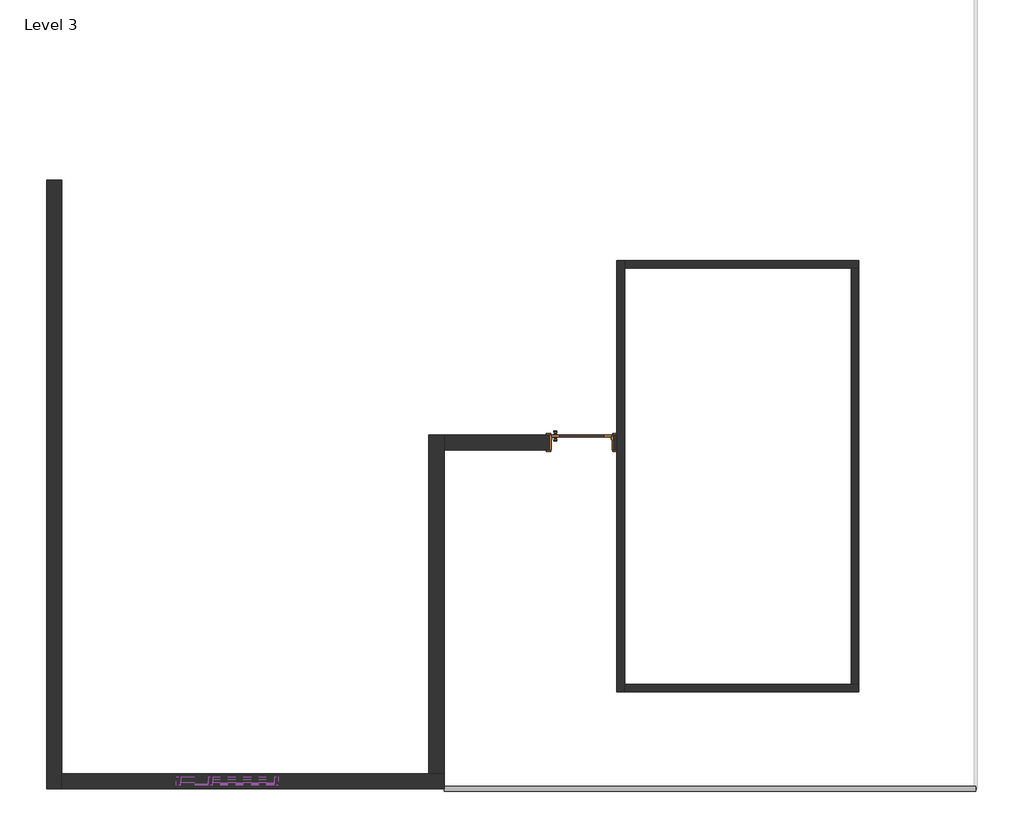
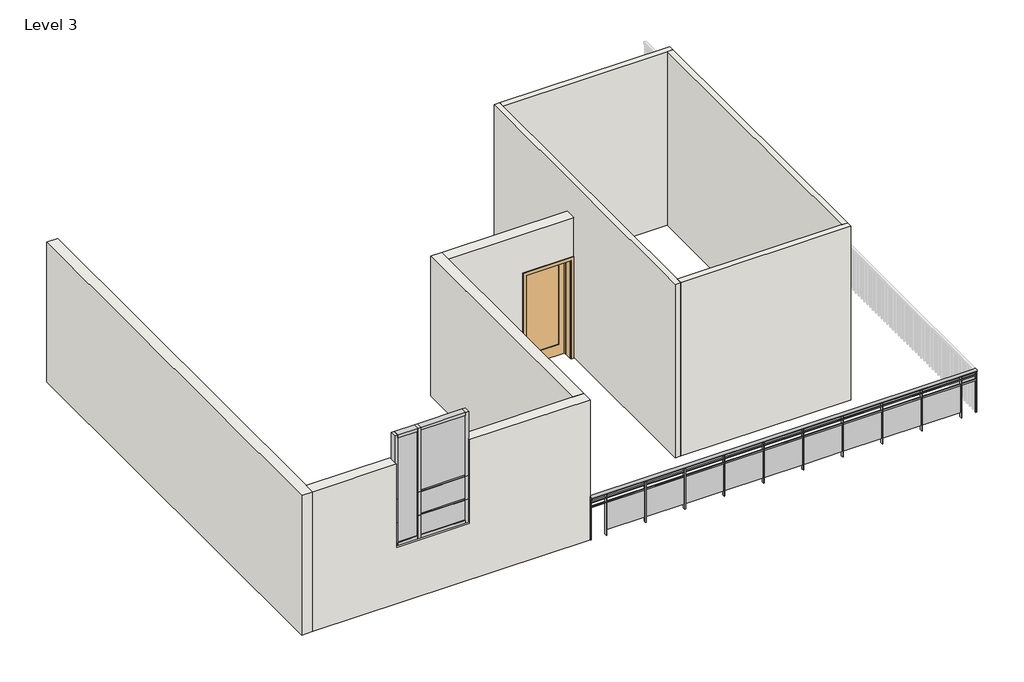
# One storey, part 1 of 2: 15 members, 8 walls, 4 plates, 1 door, 1 railing.
"""IFC4 building model written with IfcOpenShell, lengths in millimetres."""

from ifc_helpers import new_model, si_unit, point, frame, origin, place, context, project, spatial, polyline, ellipse_curve, trimmed, outline, extrude, faceted_brep, transform, mapped, element, save
from ifc_brep_helpers import plane_surface, extruded_surface, advanced_brep
from components import door_interior_single_1_panel_wood_4_x7_3b97b8e7, member_c9b54d35, member_90750a43, member_dc106669, member_ff82125d, member_7fd687a9, member_07d47f19, member_f07b7441, system_panel_glazed_5efa86ec, system_panel_glazed_31531e99, system_panel_glazed_01ea813e, system_panel_glazed_2f0fbb7d

model = new_model("IFC4")

# Units and contexts
model_context = context("Model", 3, world=origin())
ifc_project = project(units=[si_unit("LENGTHUNIT", "METRE", prefix="MILLI")], contexts=[model_context])

# Site, building, storey
site = spatial("IfcSite", under=ifc_project)
building = spatial("IfcBuilding", under=site)
storey = spatial("IfcBuildingStorey", under=building, Name="Level 3", Elevation=3810.0)

# Door
placement = place(None, origin())
door_interior_single_1_panel_wood_4_x7_shape = door_interior_single_1_panel_wood_4_x7_3b97b8e7(model_context)
element("IfcDoor", 1, ObjectType="Door-Interior-Single-1_Panel-Wood : 4'x7'", at=placement, inside=storey, context=model_context, shape_type="MappedRepresentation", body=[
    mapped(door_interior_single_1_panel_wood_4_x7_shape, transform((-360.5243879, 2041.5435469, 3810.0), x_axis=(1.0, 0.0, 0.0), y_axis=(0.0, 1.0, 0.0), z_axis=(0.0, 0.0, 1.0))),
])

# Members
member_shape = member_c9b54d35(model_context)
element("IfcMember", 2, ObjectType="Rectangular Mullion : 1.5\" x 2.5\" rectangular", at=placement, inside=storey, context=model_context, shape_type="MappedRepresentation", body=[
    mapped(member_shape, transform((-5878.6743879, -3029.0883122, 6045.2), x_axis=(0.0, 0.0, 1.0), y_axis=(0.0, 1.0, 0.0), z_axis=(-1.0, 0.0, 0.0))),
])
element("IfcMember", 3, ObjectType="Rectangular Mullion : 1.5\" x 2.5\" rectangular", at=placement, inside=storey, context=model_context, shape_type="MappedRepresentation", body=[
    mapped(member_shape, transform((-5878.6743879, -3029.0883122, 5537.2), x_axis=(0.0, 0.0, 1.0), y_axis=(0.0, 1.0, 0.0), z_axis=(-1.0, 0.0, 0.0))),
])
member_2_shape = member_90750a43(model_context)
element("IfcMember", 4, ObjectType="Rectangular Mullion : 2.5\" x 5\" rectangular", at=placement, inside=storey, context=model_context, shape_type="MappedRepresentation", body=[
    mapped(member_2_shape, transform((-5910.4243879, -3029.0883122, 5537.2), x_axis=(-1.0, 0.0, 0.0), y_axis=(0.0, 1.0, 0.0), z_axis=(0.0, 0.0, -1.0))),
])
element("IfcMember", 5, ObjectType="Rectangular Mullion : 2.5\" x 5\" rectangular", at=placement, inside=storey, context=model_context, shape_type="MappedRepresentation", body=[
    mapped(member_2_shape, transform((-5910.4243879, -3029.0883122, 5029.2), x_axis=(-1.0, 0.0, 0.0), y_axis=(0.0, 1.0, 0.0), z_axis=(0.0, 0.0, -1.0))),
])
member_3_shape = member_dc106669(model_context)
element("IfcMember", 6, ObjectType="Rectangular Mullion : 2.5\" x 5\" rectangular", at=placement, inside=storey, context=model_context, shape_type="MappedRepresentation", body=[
    mapped(member_3_shape, transform((-6354.9243879, -3029.0883122, 7442.2), x_axis=(0.0, 0.0, 1.0), y_axis=(0.0, 1.0, 0.0), z_axis=(-1.0, 0.0, 0.0))),
])
member_4_shape = member_ff82125d(model_context)
element("IfcMember", 7, ObjectType="Rectangular Mullion : 2.5\" x 5\" rectangular", at=placement, inside=storey, context=model_context, shape_type="MappedRepresentation", body=[
    mapped(member_4_shape, transform((-4957.9243879, -3029.0883122, 5029.2), x_axis=(0.0, 0.0, -1.0), y_axis=(0.0, 1.0, 0.0), z_axis=(1.0, 0.0, 0.0))),
])
element("IfcMember", 8, ObjectType="Rectangular Mullion : 2.5\" x 5\" rectangular", at=placement, inside=storey, context=model_context, shape_type="MappedRepresentation", body=[
    mapped(member_3_shape, transform((-5942.1743879, -3029.0883122, 5029.2), x_axis=(0.0, 0.0, -1.0), y_axis=(0.0, 1.0, 0.0), z_axis=(1.0, 0.0, 0.0))),
])
element("IfcMember", 9, ObjectType="Rectangular Mullion : 2.5\" x 5\" rectangular", at=placement, inside=storey, context=model_context, shape_type="MappedRepresentation", body=[
    mapped(member_4_shape, transform((-5878.6743879, -3029.0883122, 7442.2), x_axis=(0.0, 0.0, 1.0), y_axis=(0.0, 1.0, 0.0), z_axis=(-1.0, 0.0, 0.0))),
])
member_5_shape = member_7fd687a9(model_context)
element("IfcMember", 10, ObjectType="Rectangular Mullion : 2.5\" x 5\" rectangular", at=placement, inside=storey, context=model_context, shape_type="MappedRepresentation", body=[
    mapped(member_5_shape, transform((-6418.4243879, -3029.0883122, 5029.2), x_axis=(-1.0, 0.0, 0.0), y_axis=(0.0, 1.0, 0.0), z_axis=(0.0, 0.0, -1.0))),
])
element("IfcMember", 11, ObjectType="Rectangular Mullion : 2.5\" x 5\" rectangular", at=placement, inside=storey, context=model_context, shape_type="MappedRepresentation", body=[
    mapped(member_5_shape, transform((-6418.4243879, -3029.0883122, 5537.2), x_axis=(-1.0, 0.0, 0.0), y_axis=(0.0, 1.0, 0.0), z_axis=(0.0, 0.0, -1.0))),
])
element("IfcMember", 12, ObjectType="Rectangular Mullion : 2.5\" x 5\" rectangular", at=placement, inside=storey, context=model_context, shape_type="MappedRepresentation", body=[
    mapped(member_5_shape, transform((-4894.4243879, -3029.0883122, 6045.2), x_axis=(1.0, 0.0, 0.0), y_axis=(0.0, 1.0, 0.0), z_axis=(0.0, 0.0, 1.0))),
])
element("IfcMember", 13, ObjectType="Rectangular Mullion : 2.5\" x 5\" rectangular", at=placement, inside=storey, context=model_context, shape_type="MappedRepresentation", body=[
    mapped(member_5_shape, transform((-4894.4243879, -3029.0883122, 5537.2), x_axis=(1.0, 0.0, 0.0), y_axis=(0.0, 1.0, 0.0), z_axis=(0.0, 0.0, 1.0))),
])
member_6_shape = member_07d47f19(model_context)
element("IfcMember", 14, ObjectType="Rectangular Mullion : 2.5\" x 5\" rectangular", at=placement, inside=storey, context=model_context, shape_type="MappedRepresentation", body=[
    mapped(member_6_shape, transform((-5910.4243879, -3029.0883122, 6045.2), x_axis=(-1.0, 0.0, 0.0), y_axis=(0.0, 1.0, 0.0), z_axis=(0.0, 0.0, -1.0))),
])
member_7_shape = member_f07b7441(model_context)
element("IfcMember", 15, ObjectType="Rectangular Mullion : 2.5\" x 5\" rectangular", at=placement, inside=storey, context=model_context, shape_type="MappedRepresentation", body=[
    mapped(member_7_shape, transform((-4894.4243879, -3029.0883122, 7442.2), x_axis=(1.0, 0.0, 0.0), y_axis=(0.0, 1.0, 0.0), z_axis=(0.0, 0.0, 1.0))),
])
element("IfcMember", 16, ObjectType="Rectangular Mullion : 2.5\" x 5\" rectangular", at=placement, inside=storey, context=model_context, shape_type="MappedRepresentation", body=[
    mapped(member_7_shape, transform((-6418.4243879, -3029.0883122, 6045.2), x_axis=(-1.0, 0.0, 0.0), y_axis=(0.0, 1.0, 0.0), z_axis=(0.0, 0.0, -1.0))),
])

# Plates
system_panel_glazed_shape = system_panel_glazed_5efa86ec(model_context)
element("IfcPlate", 17, ObjectType="System Panel : Glazed", at=placement, inside=storey, context=model_context, shape_type="MappedRepresentation", body=[
    mapped(system_panel_glazed_shape, transform((-5418.2993879, -3029.0883122, 5092.7), x_axis=(-1.0, 0.0, 0.0), y_axis=(0.0, -1.0, 0.0), z_axis=(0.0, 0.0, 1.0))),
])
system_panel_glazed_2_shape = system_panel_glazed_31531e99(model_context)
element("IfcPlate", 18, ObjectType="System Panel : Glazed", at=placement, inside=storey, context=model_context, shape_type="MappedRepresentation", body=[
    mapped(system_panel_glazed_2_shape, transform((-5418.2993879, -3029.0883122, 5556.25), x_axis=(-1.0, 0.0, 0.0), y_axis=(0.0, -1.0, 0.0), z_axis=(0.0, 0.0, 1.0))),
])
system_panel_glazed_3_shape = system_panel_glazed_01ea813e(model_context)
element("IfcPlate", 19, ObjectType="System Panel : Glazed", at=placement, inside=storey, context=model_context, shape_type="MappedRepresentation", body=[
    mapped(system_panel_glazed_3_shape, transform((-6148.5493879, -3029.0883122, 5092.7), x_axis=(-1.0, 0.0, 0.0), y_axis=(0.0, -1.0, 0.0), z_axis=(0.0, 0.0, 1.0))),
])
system_panel_glazed_4_shape = system_panel_glazed_2f0fbb7d(model_context)
element("IfcPlate", 20, ObjectType="System Panel : Glazed", at=placement, inside=storey, context=model_context, shape_type="MappedRepresentation", body=[
    mapped(system_panel_glazed_4_shape, transform((-5418.2993879, -3029.0883122, 6064.25), x_axis=(-1.0, 0.0, 0.0), y_axis=(0.0, -1.0, 0.0), z_axis=(0.0, 0.0, 1.0))),
])

# Railing
element("IfcRailing", 21, ObjectType="Glass Panel - Bottom Fill", at=placement, inside=storey, context=model_context, shape_type="SolidModel", body=[
    advanced_brep(
    [(-2417.9243879, -3105.2883122, 4724.4), (-2417.9243879, -3181.4883122, 4724.4), (5532.2756121, -3105.2883122, 4724.4), (5532.2756121, -3181.4883122, 4724.4)],
    [
        (0, 1, ellipse_curve(frame((-2417.9243879, -3143.3883122, 4724.4), z_axis=(-1.0, 0.0, 0.0), x_axis=(0.0, -1.0, 0.0)), 38.1, 28.575)),
        (1, 0, ellipse_curve(frame((-2417.9243879, -3143.3883122, 4724.4), z_axis=(-1.0, 0.0, 0.0), x_axis=(0.0, -1.0, 0.0)), 38.1, 28.575)),
        (2, 3, ellipse_curve(frame((5532.2756121, -3143.3883122, 4724.4), z_axis=(1.0, 0.0, 0.0), x_axis=(0.0, -1.0, 0.0)), 38.1, 28.575)),
        (3, 2, ellipse_curve(frame((5532.2756121, -3143.3883122, 4724.4), z_axis=(1.0, 0.0, 0.0), x_axis=(0.0, -1.0, 0.0)), 38.1, 28.575)),
        (0, 2),
        (3, 1),
    ],
    [
        plane_surface(frame((-2417.9243879, -3143.3883122, 4724.4), z_axis=(-1.0, 0.0, 0.0), x_axis=(0.0, 1.0, 0.0))),
        plane_surface(frame((5532.2756121, -3143.3883122, 4724.4), z_axis=(1.0, 0.0, 0.0), x_axis=(0.0, 1.0, 0.0))),
        extruded_surface(trimmed(ellipse_curve(frame((5532.2756121, -3143.3883122, 4724.4), z_axis=(-1.0, 0.0, 0.0), x_axis=(0.0, -1.0, 0.0)), 38.1, 28.575), [point((5532.2756121, -3105.2883122, 4724.4))], [point((5532.2756121, -3181.4883122, 4724.4))], True, "CARTESIAN"), (-7950.200000000001, 0.0, 0.0), 7950.200000000001),
        extruded_surface(trimmed(ellipse_curve(frame((5532.2756121, -3143.3883122, 4724.4), z_axis=(-1.0, 0.0, 0.0), x_axis=(0.0, -1.0, 0.0)), 38.1, 28.575), [point((5532.2756121, -3181.4883122, 4724.4))], [point((5532.2756121, -3105.2883122, 4724.4))], True, "CARTESIAN"), (-7950.200000000001, 0.0, 0.0), 7950.200000000001),
    ],
    [
        (0, [[1, 2]]),
        (1, [[3, 4]]),
        (2, [[-1, 5, -4, 6]]),
        (3, [[-2, -6, -3, -5]]),
    ],
),
    extrude(outline(polyline([(-2417.9243879, -3156.0883122), (-2417.9243879, -3130.6883122), (5532.2756121, -3130.6883122), (5532.2756121, -3156.0883122), (-2417.9243879, -3156.0883122)])), frame((0.0, 0.0, 4610.1), z_axis=(0.0, 0.0, 1.0), x_axis=(1.0, 0.0, 0.0)), (0.0, 0.0, 1.0), 25.4),
    extrude(outline(polyline([(-2417.9243879, -3156.0883122), (-2417.9243879, -3130.6883122), (5532.2756121, -3130.6883122), (5532.2756121, -3156.0883122), (-2417.9243879, -3156.0883122)])), frame((0.0, 0.0, 4508.5), z_axis=(0.0, 0.0, 1.0), x_axis=(1.0, 0.0, 0.0)), (0.0, 0.0, 1.0), 25.4),
    extrude(outline(polyline([(5208.4256121, -3168.7883122), (5208.4256121, -3117.9883122), (5221.1256121, -3117.9883122), (5221.1256121, -3168.7883122), (5208.4256121, -3168.7883122)])), frame((0.0, 0.0, 3810.0), z_axis=(0.0, 0.0, 1.0), x_axis=(1.0, 0.0, 0.0)), (0.0, 0.0, 1.0), 885.825),
    extrude(outline(polyline([(4401.9756121, -3136.8531552), (5214.7756121, -3136.8531552), (5214.7756121, -3143.2031552), (4401.9756121, -3143.2031552), (4401.9756121, -3136.8531552)])), frame((0.0, 0.0, 3911.6), z_axis=(0.0, 0.0, 1.0), x_axis=(1.0, 0.0, 0.0)), (0.0, 0.0, 1.0), 596.9),
    extrude(outline(polyline([(4395.6256121, -3168.7883122), (4395.6256121, -3117.9883122), (4408.3256121, -3117.9883122), (4408.3256121, -3168.7883122), (4395.6256121, -3168.7883122)])), frame((0.0, 0.0, 3810.0), z_axis=(0.0, 0.0, 1.0), x_axis=(1.0, 0.0, 0.0)), (0.0, 0.0, 1.0), 885.825),
    extrude(outline(polyline([(3589.1756121, -3136.8531552), (4401.9756121, -3136.8531552), (4401.9756121, -3143.2031552), (3589.1756121, -3143.2031552), (3589.1756121, -3136.8531552)])), frame((0.0, 0.0, 3911.6), z_axis=(0.0, 0.0, 1.0), x_axis=(1.0, 0.0, 0.0)), (0.0, 0.0, 1.0), 596.9),
    extrude(outline(polyline([(3582.8256121, -3168.7883122), (3582.8256121, -3117.9883122), (3595.5256121, -3117.9883122), (3595.5256121, -3168.7883122), (3582.8256121, -3168.7883122)])), frame((0.0, 0.0, 3810.0), z_axis=(0.0, 0.0, 1.0), x_axis=(1.0, 0.0, 0.0)), (0.0, 0.0, 1.0), 885.825),
    extrude(outline(polyline([(2776.3756121, -3136.8531552), (3589.1756121, -3136.8531552), (3589.1756121, -3143.2031552), (2776.3756121, -3143.2031552), (2776.3756121, -3136.8531552)])), frame((0.0, 0.0, 3911.6), z_axis=(0.0, 0.0, 1.0), x_axis=(1.0, 0.0, 0.0)), (0.0, 0.0, 1.0), 596.9),
    extrude(outline(polyline([(2770.0256121, -3168.7883122), (2770.0256121, -3117.9883122), (2782.7256121, -3117.9883122), (2782.7256121, -3168.7883122), (2770.0256121, -3168.7883122)])), frame((0.0, 0.0, 3810.0), z_axis=(0.0, 0.0, 1.0), x_axis=(1.0, 0.0, 0.0)), (0.0, 0.0, 1.0), 885.825),
    extrude(outline(polyline([(1963.5756121, -3136.8531552), (2776.3756121, -3136.8531552), (2776.3756121, -3143.2031552), (1963.5756121, -3143.2031552), (1963.5756121, -3136.8531552)])), frame((0.0, 0.0, 3911.6), z_axis=(0.0, 0.0, 1.0), x_axis=(1.0, 0.0, 0.0)), (0.0, 0.0, 1.0), 596.9),
    extrude(outline(polyline([(1957.2256121, -3168.7883122), (1957.2256121, -3117.9883122), (1969.9256121, -3117.9883122), (1969.9256121, -3168.7883122), (1957.2256121, -3168.7883122)])), frame((0.0, 0.0, 3810.0), z_axis=(0.0, 0.0, 1.0), x_axis=(1.0, 0.0, 0.0)), (0.0, 0.0, 1.0), 885.825),
    extrude(outline(polyline([(1150.7756121, -3136.8531552), (1963.5756121, -3136.8531552), (1963.5756121, -3143.2031552), (1150.7756121, -3143.2031552), (1150.7756121, -3136.8531552)])), frame((0.0, 0.0, 3911.6), z_axis=(0.0, 0.0, 1.0), x_axis=(1.0, 0.0, 0.0)), (0.0, 0.0, 1.0), 596.9),
    extrude(outline(polyline([(1144.4256121, -3168.7883122), (1144.4256121, -3117.9883122), (1157.1256121, -3117.9883122), (1157.1256121, -3168.7883122), (1144.4256121, -3168.7883122)])), frame((0.0, 0.0, 3810.0), z_axis=(0.0, 0.0, 1.0), x_axis=(1.0, 0.0, 0.0)), (0.0, 0.0, 1.0), 885.825),
    extrude(outline(polyline([(337.9756121, -3136.8531552), (1150.7756121, -3136.8531552), (1150.7756121, -3143.2031552), (337.9756121, -3143.2031552), (337.9756121, -3136.8531552)])), frame((0.0, 0.0, 3911.6), z_axis=(0.0, 0.0, 1.0), x_axis=(1.0, 0.0, 0.0)), (0.0, 0.0, 1.0), 596.9),
    extrude(outline(polyline([(331.6256121, -3168.7883122), (331.6256121, -3117.9883122), (344.3256121, -3117.9883122), (344.3256121, -3168.7883122), (331.6256121, -3168.7883122)])), frame((0.0, 0.0, 3810.0), z_axis=(0.0, 0.0, 1.0), x_axis=(1.0, 0.0, 0.0)), (0.0, 0.0, 1.0), 885.825),
    extrude(outline(polyline([(-474.8243879, -3136.8531552), (337.9756121, -3136.8531552), (337.9756121, -3143.2031552), (-474.8243879, -3143.2031552), (-474.8243879, -3136.8531552)])), frame((0.0, 0.0, 3911.6), z_axis=(0.0, 0.0, 1.0), x_axis=(1.0, 0.0, 0.0)), (0.0, 0.0, 1.0), 596.9),
    extrude(outline(polyline([(-481.1743879, -3168.7883122), (-481.1743879, -3117.9883122), (-468.4743879, -3117.9883122), (-468.4743879, -3168.7883122), (-481.1743879, -3168.7883122)])), frame((0.0, 0.0, 3810.0), z_axis=(0.0, 0.0, 1.0), x_axis=(1.0, 0.0, 0.0)), (0.0, 0.0, 1.0), 885.825),
    extrude(outline(polyline([(-1287.6243879, -3136.8531552), (-474.8243879, -3136.8531552), (-474.8243879, -3143.2031552), (-1287.6243879, -3143.2031552), (-1287.6243879, -3136.8531552)])), frame((0.0, 0.0, 3911.6), z_axis=(0.0, 0.0, 1.0), x_axis=(1.0, 0.0, 0.0)), (0.0, 0.0, 1.0), 596.9),
    extrude(outline(polyline([(-1293.9743879, -3168.7883122), (-1293.9743879, -3117.9883122), (-1281.2743879, -3117.9883122), (-1281.2743879, -3168.7883122), (-1293.9743879, -3168.7883122)])), frame((0.0, 0.0, 3810.0), z_axis=(0.0, 0.0, 1.0), x_axis=(1.0, 0.0, 0.0)), (0.0, 0.0, 1.0), 885.825),
    extrude(outline(polyline([(-2100.4243879, -3136.8531552), (-1287.6243879, -3136.8531552), (-1287.6243879, -3143.2031552), (-2100.4243879, -3143.2031552), (-2100.4243879, -3136.8531552)])), frame((0.0, 0.0, 3911.6), z_axis=(0.0, 0.0, 1.0), x_axis=(1.0, 0.0, 0.0)), (0.0, 0.0, 1.0), 596.9),
    extrude(outline(polyline([(-2106.7743879, -3168.7883122), (-2106.7743879, -3117.9883122), (-2094.0743879, -3117.9883122), (-2094.0743879, -3168.7883122), (-2106.7743879, -3168.7883122)])), frame((0.0, 0.0, 3810.0), z_axis=(0.0, 0.0, 1.0), x_axis=(1.0, 0.0, 0.0)), (0.0, 0.0, 1.0), 885.825),
    extrude(outline(polyline([(5519.5756121, -3152.9133122), (5519.5756121, -3133.8633122), (5538.6256121, -3133.8633122), (5538.6256121, -3152.9133122), (5519.5756121, -3152.9133122)])), frame((0.0, 0.0, 3810.0), z_axis=(0.0, 0.0, 1.0), x_axis=(1.0, 0.0, 0.0)), (0.0, 0.0, 1.0), 885.825),
    extrude(outline(polyline([(-2424.2743879, -3152.9133122), (-2424.2743879, -3133.8633122), (-2405.2243879, -3133.8633122), (-2405.2243879, -3152.9133122), (-2424.2743879, -3152.9133122)])), frame((0.0, 0.0, 3810.0), z_axis=(0.0, 0.0, 1.0), x_axis=(1.0, 0.0, 0.0)), (0.0, 0.0, 1.0), 885.825),
])

# Walls
element("IfcWall", 22, ObjectType="4.5\" wall", at=placement, inside=storey, context=model_context, shape_type="Brep", body=[
    faceted_brep([(280.8256121, -1695.4314531, 3810.0), (280.8256121, -1581.1314531, 3810.0), (280.8256121, 4648.2185469, 3810.0), (280.8256121, 4762.5185469, 3810.0), (280.8256121, 4762.5185469, 7594.6), (280.8256121, 4648.2185469, 7594.6), (280.8256121, -1581.1314531, 7594.6), (280.8256121, -1695.4314531, 7594.6), (166.5256121, -1695.4314531, 3810.0), (166.5256121, -1695.4314531, 7594.6), (166.5256121, 4762.5185469, 7594.6), (166.5256121, 4762.5185469, 3810.0), (166.5256121, 2152.6685469, 3810.0), (166.5256121, 1924.0685469, 3810.0)], [[[0, 1, 2, 3, 4, 5, 6, 7]], [[8, 9, 10, 11, 12, 13]], [[3, 2, 1, 0, 8, 13, 12, 11]], [[7, 6, 5, 4, 10, 9]], [[0, 7, 9, 8]], [[4, 3, 11, 10]]]),
])
element("IfcWall", 23, ObjectType="4.5\" wall", at=placement, inside=storey, context=model_context, shape_type="Brep", body=[
    faceted_brep([(3786.0256121, -1581.1314531, 3810.0), (3671.7256121, -1581.1314531, 3810.0), (280.8256121, -1581.1314531, 3810.0), (280.8256121, -1581.1314531, 7594.6), (3671.7256121, -1581.1314531, 7594.6), (3786.0256121, -1581.1314531, 7594.6), (3786.0256121, -1695.4314531, 3810.0), (3786.0256121, -1695.4314531, 7594.6), (280.8256121, -1695.4314531, 7594.6), (280.8256121, -1695.4314531, 3810.0)], [[[0, 1, 2, 3, 4, 5]], [[6, 7, 8, 9]], [[2, 1, 0, 6, 9]], [[5, 4, 3, 8, 7]], [[0, 5, 7, 6]], [[3, 2, 9, 8]]]),
])
element("IfcWall", 24, ObjectType="4.5\" wall", at=placement, inside=storey, context=model_context, shape_type="SweptSolid", body=[
    extrude(outline(polyline([(3671.7256121, -1581.1314531), (3671.7256121, 4648.2185469), (3786.0256121, 4648.2185469), (3786.0256121, -1581.1314531), (3671.7256121, -1581.1314531)])), frame((0.0, 0.0, 3810.0), z_axis=(0.0, 0.0, 1.0), x_axis=(1.0, 0.0, 0.0)), (0.0, 0.0, 1.0), 3784.6),
])
element("IfcWall", 25, ObjectType="4.5\" wall", at=placement, inside=storey, context=model_context, shape_type="Brep", body=[
    faceted_brep([(280.8256121, 4648.2185469, 3810.0), (3671.7256121, 4648.2185469, 3810.0), (3786.0256121, 4648.2185469, 3810.0), (3786.0256121, 4648.2185469, 7594.6), (3671.7256121, 4648.2185469, 7594.6), (280.8256121, 4648.2185469, 7594.6), (280.8256121, 4762.5185469, 3810.0), (280.8256121, 4762.5185469, 7594.6), (3786.0256121, 4762.5185469, 7594.6), (3786.0256121, 4762.5185469, 3810.0)], [[[0, 1, 2, 3, 4, 5]], [[6, 7, 8, 9]], [[2, 1, 0, 6, 9]], [[5, 4, 3, 8, 7]], [[0, 5, 7, 6]], [[3, 2, 9, 8]]]),
])
element("IfcWall", 26, ObjectType="9\" wall", at=placement, inside=storey, context=model_context, shape_type="Brep", body=[
    faceted_brep([(-8361.5243879, 5962.5116878, 3810.0), (-8361.5243879, -3143.3883122, 3810.0), (-8361.5243879, -3143.3883122, 6858.0), (-8361.5243879, 5962.5116878, 6858.0), (-8132.9243879, 5962.5116878, 3810.0), (-8132.9243879, 5962.5116878, 6858.0), (-8132.9243879, -2914.7883122, 6858.0), (-8132.9243879, -3143.3883122, 6858.0), (-8132.9243879, -3143.3883122, 3810.0), (-8132.9243879, -2914.7883122, 3810.0)], [[[0, 1, 2, 3]], [[4, 5, 6, 7, 8, 9]], [[1, 0, 4, 9, 8]], [[3, 2, 7, 6, 5]], [[0, 3, 5, 4]], [[2, 1, 8, 7]]]),
])
element("IfcWall", 27, ObjectType="9\" wall", at=placement, inside=storey, context=model_context, shape_type="Brep", body=[
    faceted_brep([(-8132.9243879, -3143.3883122, 3810.0), (-2417.9243879, -3143.3883122, 3810.0), (-2417.9243879, -3143.3883122, 6858.0), (-4894.4243879, -3143.3883122, 6858.0), (-4894.4243879, -3143.3883122, 5029.2), (-6418.4243879, -3143.3883122, 5029.2), (-6418.4243879, -3143.3883122, 6858.0), (-8132.9243879, -3143.3883122, 6858.0), (-2417.9243879, -2914.7883122, 3810.0), (-2646.5243879, -2914.7883122, 3810.0), (-8132.9243879, -2914.7883122, 3810.0), (-8132.9243879, -2914.7883122, 6858.0), (-6418.4243879, -2914.7883122, 6858.0), (-6418.4243879, -2914.7883122, 5029.2), (-4894.4243879, -2914.7883122, 5029.2), (-4894.4243879, -2914.7883122, 6858.0), (-2646.5243879, -2914.7883122, 6858.0), (-2417.9243879, -2914.7883122, 6858.0)], [[[0, 1, 2, 3, 4, 5, 6, 7]], [[8, 9, 10, 11, 12, 13, 14, 15, 16, 17]], [[1, 0, 10, 9, 8]], [[11, 7, 6, 12]], [[2, 17, 16, 15, 3]], [[0, 7, 11, 10]], [[2, 1, 8, 17]], [[14, 4, 3, 15]], [[5, 13, 12, 6]], [[4, 14, 13, 5]]]),
])
element("IfcWall", 28, ObjectType="9\" wall", at=placement, inside=storey, context=model_context, shape_type="Brep", body=[
    faceted_brep([(-2417.9243879, -2914.7883122, 3810.0), (-2417.9243879, 1924.0685469, 3810.0), (-2417.9243879, 2152.6685469, 3810.0), (-2417.9243879, 2152.6685469, 6858.0), (-2417.9243879, 1924.0685469, 6858.0), (-2417.9243879, -2914.7883122, 6858.0), (-2646.5243879, -2914.7883122, 3810.0), (-2646.5243879, -2914.7883122, 6858.0), (-2646.5243879, 2152.6685469, 6858.0), (-2646.5243879, 2152.6685469, 3810.0)], [[[0, 1, 2, 3, 4, 5]], [[6, 7, 8, 9]], [[2, 1, 0, 6, 9]], [[5, 4, 3, 8, 7]], [[0, 5, 7, 6]], [[3, 2, 9, 8]]]),
])
element("IfcWall", 29, ObjectType="9\" wall", at=placement, inside=storey, context=model_context, shape_type="SweptSolid", body=[
    extrude(outline(polyline([(6858.0, 166.5256121), (6858.0, -2417.9243879), (3810.0, -2417.9243879), (3810.0, -843.1243879), (5969.0, -843.1243879), (5969.0, 122.0756121), (3810.0, 122.0756121), (3810.0, 166.5256121), (6858.0, 166.5256121)])), frame((0.0, 1924.0685469, 0.0), z_axis=(0.0, 1.0, 0.0), x_axis=(0.0, 0.0, 1.0)), (0.0, 0.0, 1.0), 228.6),
])

save(model, "model.ifc")

# Revit data of these elements
# Type "Door-Interior-Single-1_Panel-Wood : 4'x7'"
#   Type Mark = "9"
#   Assembly Code = "C1020300"
#   Analytic Construction = "Wooden"
#   Top Rail = 0' - 4 11/16"
#   Thickness = 0' - 1 3/8"
#   Thermal Resistance (R) = 2.5876 (h·ft²·°F)/BTU
#   Swing Angle [instance default] = 90.00°
#   Stiles = 0' - 4 3/4"
#   Rough Width = 3' - 2"
#   Rough Height = 7' - 1"
#   Height = 7' - 0"
#   Width = 3' - 0"
#   Heat Transfer Coefficient (U) = 0.3865 BTU/(h·ft²·°F)
#   Bottom Rail = 0' - 9 1/8"
#   Trim Material = Cherry
#   Panel Material = Cherry
#   Frame Material = Cherry
#   Door Handle Material = Aluminum
#   Visual Light Transmittance = 0
#   Solar Heat Gain Coefficient = 0
#   Wall Closure = (empty or 0)
#   Function = (empty or 0)
# Type "Rectangular Mullion : 1.5\" x 2.5\" rectangular"
#   built-in parameter 1007304 = 0.208333 (stored number, unit not read)
#   built-in parameter 1007301 = 0.0625 (stored number, unit not read)
#   built-in parameter 1007300 = 0.0625 (stored number, unit not read)
# Type "Rectangular Mullion : 2.5\" x 5\" rectangular"
#   built-in parameter 1007304 = 0.416667 (stored number, unit not read)
#   built-in parameter 1007301 = 0.104167 (stored number, unit not read)
#   built-in parameter 1007300 = 0.104167 (stored number, unit not read)
# Type "System Panel : Glazed"
#   Construction Type Id = "GSP4R"
#   Analytic Construction = "1/8 in Pilkington single glazing"
#   Visual Light Transmittance = 0.9
#   Solar Heat Gain Coefficient = 0.86
#   Heat Transfer Coefficient (U) = 1.18115 BTU/(h·ft²·°F)
#   Define Thermal Properties by = 1
# Type "Glass Panel - Bottom Fill"
#   Assembly Code = "C2010400"
#   built-in parameter 1008612 = 0.0416667 (stored number, unit not read)
#   built-in parameter 1008611 = 0.0416667 (stored number, unit not read)
#   built-in parameter 1008609 = 0.333333 (stored number, unit not read)
#   built-in parameter 1008604 = 0.166667 (stored number, unit not read)
#   built-in parameter 1008603 = 0.166667 (stored number, unit not read)
#   Railing Height = 3' - 0"
#   built-in parameter 1008630 = 2
#   built-in parameter 1008610 = 2
#   built-in parameter 1008618 = Baluster - Square : 3/4"
# Type "4.5\" wall"
#   Assembly Code = "B2010"
#   Layers, outside or top first: 0' - 4 1/2" no material (function 1)
# Type "9\" wall"
#   Assembly Code = "B2010"
#   Layers, outside or top first: 0' - 9" no material (function 1)
# Element 1 (IfcDoor, "Door-Interior-Single-1_Panel-Wood : 4'x7'")
#   Swing Angle = 90.00°
#   Phase Created = New Construction
#   Materials on its faces: "Cherry", "Aluminum"
# Elements 2, 3 (IfcMember, "Rectangular Mullion : 1.5\" x 2.5\" rectangular")
#   Phase Created = New Construction
# Elements 4, 5, 6, 7, 8, 9, 10, 11, 12, 13, 14, 15, 16 (IfcMember, "Rectangular Mullion : 2.5\" x 5\" rectangular")
#   Phase Created = New Construction
# Elements 17, 18, 19, 20 (IfcPlate, "System Panel : Glazed")
#   Phase Created = New Construction
#   Materials on its faces: "Glass"
# Element 21 (IfcRailing, "Glass Panel - Bottom Fill")
#   Phase Created = New Construction
#   Materials on its faces: "Glass"
# Elements 22, 23, 24, 25 (IfcWall, "4.5\" wall")
#   Top Offset = -1' - 0"
#   Base Offset = 0' - 0"
#   wall height = 12' - 5"
#   Phase Created = New Construction
#   Base Constraint = Level 3
#   Top Constraint = Level 5
#   Materials on its faces: "Default Wall"
# Elements 26, 27, 28, 29 (IfcWall, "9\" wall")
#   Top Offset = 0' - 0"
#   Base Offset = 0' - 0"
#   wall height = 10' - 0"
#   Phase Created = New Construction
#   Base Constraint = Level 3
#   Top Constraint = Level 4
#   Materials on its faces: "Default Wall"
# Materials
#   "Cherry": class "Wood", colour RGB 226 177 128, transparency 0, Description = "Prunus Serotina", Cost = 0
#   "Aluminum": class "Metal", colour RGB 247 247 247, transparency 0, Description = "Aluminum 6061", Cost = 0
#   "Glass": class "Glass", colour RGB 0 128 192, transparency 0.75, Description = "Soda Lime Glass", Cost = 0
#   "Default Wall": colour RGB 128 128 128, transparency 0, Cost = 0
